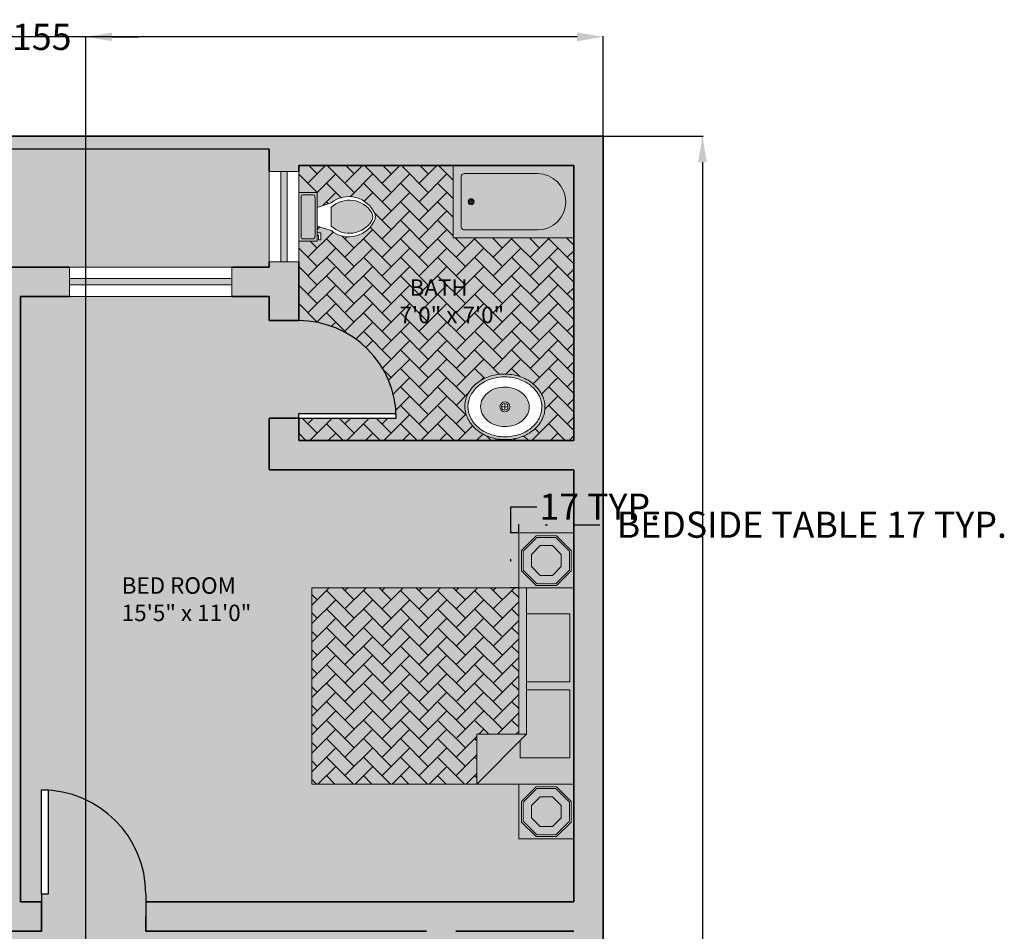
# Model space of a CAD drawing. Units: inches. Extents: x 389 to 971, y 148 to 870.
# Tile 14 of 14: x 670 to 971, y 592 to 870. Entities that reach past the tile are written whole.
import ezdxf

# ---------------------------------------------------------------- set-up
doc = ezdxf.new("R2010")
doc.units = ezdxf.units.IN
doc.header["$MEASUREMENT"] = 0
for name, color, linetype, lineweight in [('A-ANNO-DIMS', 2, 'Continuous', 18), ('A-AREA-IDEN', 7, 'Continuous', 18), ('A-DOOR', 4, 'Continuous', 25), ('A-FLOR-BASE-PATT', 8, 'Continuous', 13), ('A-FLOR-FIXT', 8, 'Continuous', 18), ('A-FLOR-FIXT-PATT', 9, 'Continuous', 13), ('A-FLOR-PATT', 9, 'Continuous', 13), ('A-FURN', 8, 'Continuous', 18), ('A-FURN-PATT', 8, 'Continuous', 13), ('A-GLAZ', 4, 'Continuous', 18), ('A-WALL', 7, 'Continuous', 35), ('C-PROP', 7, 'Continuous', 35), ('L-GRND-BASE-PATT', 8, 'Continuous', 13), ('L-WALL', 7, 'Continuous', 30)]:
    doc.layers.add(name, color=color, linetype=linetype, lineweight=lineweight)
for name, color, linetype, lineweight, true_color in [('A-FURN-SURF-PATT', 9, 'Continuous', 13, 0xd6bdce), ('A-GLAZ-PATT', 251, 'Continuous', 13, 0x6d5f6c), ('A-WALL-PATT', 18, 'Continuous', 13, 0x000000), ('L-GRND-PATT', 39, 'Continuous', 13, 0x603913)]:
    doc.layers.add(name, color=color, linetype=linetype, lineweight=lineweight, true_color=true_color)
doc.styles.get("Standard").update_dxf_attribs({"font": 'arial.ttf'})
doc.dimstyles.get("Standard").update_dxf_attribs({"dimtxt": 8, "dimasz": 8, "dimexe": 0.18, "dimexo": 0.0625, "dimgap": 0.09, "dimtad": 0, "dimtih": 1, "dimtoh": 1, "dimdec": 0, "dimzin": 0, "dimdsep": 46, "dimlunit": 3, "dimtxsty": 'Standard', "dimcen": 0.09, "dimadec": 0, "dimazin": 0, "dimtfac": 1, "dimtdec": 0, "dimtofl": 0, "dimtmove": 0, "dimatfit": 3, "dimfxl": 1, "dimtolj": 1, "dimtzin": 0, "dimarcsym": 0})

# ---------------------------------------------------------------- blocks, each defined once
blk = doc.blocks.new('*U5')
for p, q in [((0, 0), (0, -6)), ((28, 0), (28, -6))]:
    blk.add_line(p, q)
blk.add_lwpolyline([(0, 0), (0, 28), (1.75, 28), (1.75, 0)], close=True)
blk.add_arc((0, 0), 28, 0, 90)
blk = doc.blocks.new('*U3')
for p, q in [((0, 0), (0, -6)), ((-40, 0), (-40, -6))]:
    blk.add_line(p, q)
blk.add_lwpolyline([(0, 0), (0, 40), (-1.75, 40), (-1.75, 0)], close=True)
blk.add_arc((0, 0), 40, 90, 180)
blk = doc.blocks.new('Hot Tub')
for p, q in [((0, 0), (0, 69.12)), ((0, 69.12), (69.12, 69.12)), ((21.601, 65.456), (3.272, 47.128)), ((22.464, 63.396), (5.358, 46.29)), ((47.521, 65.456), (21.601, 65.456)), ((46.656, 63.396), (22.464, 63.396)), ((63.763, 46.29), (46.656, 63.396)), ((65.849, 47.128), (47.521, 65.456)), ((69.12, 69.12), (69.12, 0)), ((26.785, 53.097), (15.788, 42.101)), ((42.337, 53.097), (26.785, 53.097)), ((53.333, 42.101), (42.337, 53.097)), ((3.272, 47.128), (3.272, 21.208)), ((5.358, 46.29), (5.358, 22.098)), ((15.788, 42.101), (15.788, 26.549)), ((53.333, 26.549), (53.333, 42.101)), ((63.763, 22.098), (63.763, 46.29)), ((65.849, 21.208), (65.849, 47.128)), ((15.788, 26.549), (26.785, 15.552)), ((42.337, 15.552), (53.333, 26.549)), ((3.272, 21.208), (21.601, 2.88)), ((5.358, 22.098), (22.464, 4.992)), ((26.785, 15.552), (42.337, 15.552)), ((46.656, 4.992), (63.763, 22.098)), ((47.521, 2.88), (65.849, 21.208)), ((69.12, 0), (0, 0)), ((21.601, 2.88), (47.521, 2.88)), ((22.464, 4.992), (46.656, 4.992))]:
    blk.add_line(p, q)
blk = doc.blocks.new('Toilet - top')
for p, q in [((9.5, -6), (9.5, -2)), ((-8, -8.5), (-8, -8)), ((-7, -8), (-7, -9.5)), ((-4, -8), (-6, -14)), ((4, -8), (6, -14)), ((-10, -8.5), (-8, -8.5)), ((-10, -9.5), (-10, -8.5)), ((-7, -9.5), (-10, -9.5)), ((4, -14), (-4, -14))]:
    blk.add_line(p, q)
blk.add_lwpolyline([(10.5, -8), (10.5, 0), (-10.5, 0), (-10.5, -8)], close=True)
for points in [[(-9.5, -2), (-9.5, -6)], [(8.5, -1), (-8.5, -1)], [(-8.5, -7), (8.5, -7)]]:
    blk.add_lwpolyline(points)
for centre, radius, start, end in [((-8.62, -1.88), 0.884, 81.8699, 188.1301), ((8.62, -1.88), 0.884, 351.8699, 98.1301), ((-8.62, -6.12), 0.884, 171.8699, 278.1301), ((8.62, -6.12), 0.884, 261.8699, 8.1301), ((3.52, -21.58), 12.17, 141.4691, 247.9714), ((4.2, -21.82), 11.33, 136.3677, 238.9468), ((-3.52, -21.58), 12.17, 292.0284, 38.5307), ((-4.2, -21.82), 11.33, 301.053, 43.6321), ((0, -27.88), 4, 245.7318, 294.2682), ((0, -29), 4, 254.8605, 285.1395)]:
    blk.add_arc(centre, radius, start, end)
blk = doc.blocks.new('Bed - Queen')
for p, q in [((0, -80.00003), (0, 0)), ((0, 0), (59.99999, 0)), ((59.99999, 0), (59.99999, -80.00003)), ((7.99999, -1.2), (28.79998, -1.2)), ((7.99999, -14.4), (7.99999, -1.2)), ((28.79998, -1.2), (28.79998, -14.4)), ((31.19999, -1.2), (51.99999, -1.2)), ((31.19999, -14.4), (31.19999, -1.2)), ((51.99999, -1.2), (51.99999, -16.4)), ((0, -14.4), (44.8, -14.4)), ((59.99999, -29.6), (44.8, -14.4)), ((44.8, -14.4), (44.8, -29.6)), ((44.8, -16.8), (0, -16.8)), ((51.99999, -16.4), (46.79936, -16.4)), ((44.8, -29.6), (59.99999, -29.6)), ((59.99999, -80.00003), (0, -80.00003))]:
    blk.add_line(p, q)
blk = doc.blocks.new('Sink - Oval top')
for p, q in [((-1, 0), (1, 0)), ((0, 1), (0, -1))]:
    blk.add_line(p, q)
for points in [[(-12.23, 0.39, 0.117634), (-11.46, -3.36, 0.104469), (-8.88, -6.8, 0.090016), (-5.08, -9.07, 0.08192), (-0.32, -10.02, 0.08192), (4.49, -9.38, 0.090016), (8.42, -7.36, 0.104469), (11.22, -4.09, 0.117634), (12.23, -0.39, 0.117634), (11.46, 3.36, 0.104469), (8.88, 6.8, 0.090016), (5.08, 9.07, 0.08192), (0.32, 10.02, 0.08192), (-4.49, 9.38, 0.090016), (-8.42, 7.36, 0.104469), (-11.22, 4.09, 0.117634)], [(-11.29, 0.16, 0.118622), (-10.52, -3.25, 0.104678), (-8.07, -6.36, 0.089562), (-4.54, -8.37, 0.081185), (-0.13, -9.15, 0.081185), (4.3, -8.49, 0.089562), (7.89, -6.58, 0.104678), (10.42, -3.55, 0.118622), (11.29, -0.16, 0.118622), (10.52, 3.25, 0.104678), (8.07, 6.36, 0.089562), (4.54, 8.37, 0.081185), (0.13, 9.15, 0.081185), (-4.3, 8.49, 0.089562), (-7.89, 6.58, 0.104678), (-10.42, 3.55, 0.118622)], [(-7.42, 0.08, 0.118283), (-6.91, -2.17, 0.104607), (-5.29, -4.21, 0.089718), (-2.97, -5.53, 0.081436), (-0.07, -6.04, 0.081436), (2.84, -5.59, 0.089718), (5.2, -4.33, 0.104607), (6.86, -2.32, 0.118283), (7.42, -0.08, 0.118283), (6.91, 2.17, 0.104607), (5.29, 4.21, 0.089718), (2.97, 5.53, 0.081436), (0.07, 6.04, 0.081436), (-2.84, 5.59, 0.089718), (-5.2, 4.33, 0.104607), (-6.86, 2.32, 0.118283)]]:
    blk.add_lwpolyline(points, format="xyb", close=True)
for radius in [1.5, 1]:
    blk.add_circle((0, 0), radius)
blk = doc.blocks.new('Bath Tub - 26 x 60 in.')
for p, q in [((8, -18), (10, -18)), ((9, -17), (9, -19))]:
    blk.add_line(p, q)
blk.add_lwpolyline([(0, -36), (0, 0), (60, 0), (60, -36)], close=True)
for points in [[(6, -4), (42, -4)], [(4, -30), (4, -6)], [(42, -32), (6, -32)]]:
    blk.add_lwpolyline(points)
for radius in [1.5, 1]:
    blk.add_circle((9, -18), radius)
for centre, radius, start, end in [((5.75, -5.75), 1.77, 81.8699, 188.1301), ((42, -18), 14, 270, 90), ((5.75, -30.25), 1.77, 171.8699, 278.1301)]:
    blk.add_arc(centre, radius, start, end)
blk = doc.blocks.new('*D22')
at = {"layer": 'A-ANNO-DIMS', "color": 0, "lineweight": -2, "transparency": 16777216}
for p, q in [((822.48, 713.45), (822.48, 716.08)), ((830.48, 715.9), (831.22, 715.9)), ((839.22, 713.45), (839.22, 716.08)), ((839.22, 715.9), (847.22, 715.9))]:
    blk.add_line(p, q, dxfattribs=at)
at = {"layer": 'A-ANNO-DIMS', "color": 0, "transparency": 16777216}
for points in [[(830.48, 717.23), (830.48, 714.56), (822.48, 715.9)], [(831.22, 717.23), (831.22, 714.56), (839.22, 715.9)]]:
    blk.add_solid(points, dxfattribs=at)
at = {"layer": 'Defpoints', "color": 0, "transparency": 16777216}
for p in [(839.22, 715.9), (822.48, 713.39), (839.22, 713.39)]:
    blk.add_point(p, dxfattribs=at)
at = {"layer": 'A-ANNO-DIMS', "color": 0, "transparency": 16777216, "insert": (911.94, 715.9), "char_height": 8, "attachment_point": 5}
blk.add_mtext('\\A1;BEDSIDE TABLE 17 TYP.', dxfattribs=at)
blk = doc.blocks.new('*D23')
at = {"layer": 'A-ANNO-DIMS', "color": 0, "lineweight": -2, "transparency": 16777216}
for p, q in [((819.96, 713.39), (819.96, 721.39)), ((819.96, 721.39), (827.96, 721.39)), ((822.41, 713.39), (819.78, 713.39)), ((819.96, 704.64), (819.96, 705.39)), ((822.41, 696.64), (819.78, 696.64))]:
    blk.add_line(p, q, dxfattribs=at)
at = {"layer": 'A-ANNO-DIMS', "color": 0, "transparency": 16777216}
for points in [[(818.63, 705.39), (821.3, 705.39), (819.96, 713.39)], [(818.63, 704.64), (821.3, 704.64), (819.96, 696.64)]]:
    blk.add_solid(points, dxfattribs=at)
at = {"layer": 'Defpoints', "color": 0, "transparency": 16777216}
for p in [(819.96, 713.39), (822.48, 713.39), (822.48, 696.64)]:
    blk.add_point(p, dxfattribs=at)
at = {"layer": 'A-ANNO-DIMS', "color": 0, "transparency": 16777216, "insert": (847.15, 721.39), "char_height": 8, "attachment_point": 5}
blk.add_mtext('\\A1;17 TYP.', dxfattribs=at)
blk = doc.blocks.new('*D46')
at = {"layer": 'A-ANNO-DIMS', "color": 0, "lineweight": -2, "transparency": 16777216}
for p, q in [((468.22, 794.71), (468.22, 865.15)), ((476.22, 864.97), (649.3, 864.97)), ((840.22, 864.97), (667.13, 864.97)), ((848.22, 834.71), (848.22, 865.15))]:
    blk.add_line(p, q, dxfattribs=at)
at = {"layer": 'A-ANNO-DIMS', "color": 0, "transparency": 16777216}
for points in [[(476.22, 866.3), (476.22, 863.64), (468.22, 864.97)], [(840.22, 866.3), (840.22, 863.64), (848.22, 864.97)]]:
    blk.add_solid(points, dxfattribs=at)
at = {"layer": 'Defpoints', "color": 0, "transparency": 16777216}
for p in [(848.22, 864.97), (848.22, 834.64), (468.22, 794.64)]:
    blk.add_point(p, dxfattribs=at)
at = {"layer": 'A-ANNO-DIMS', "color": 0, "transparency": 16777216, "insert": (658.22, 864.97), "char_height": 8, "attachment_point": 5}
blk.add_mtext('\\A1;380', dxfattribs=at)
blk = doc.blocks.new('*D47')
at = {"layer": 'A-ANNO-DIMS', "color": 0, "lineweight": -2, "transparency": 16777216}
for p, q in [((848.28, 834.64), (878.72, 834.64)), ((878.54, 826.64), (878.54, 564.32)), ((878.54, 293.64), (878.54, 555.97)), ((839.28, 285.64), (878.72, 285.64))]:
    blk.add_line(p, q, dxfattribs=at)
at = {"layer": 'A-ANNO-DIMS', "color": 0, "transparency": 16777216}
for points in [[(877.21, 826.64), (879.87, 826.64), (878.54, 834.64)], [(877.21, 293.64), (879.87, 293.64), (878.54, 285.64)]]:
    blk.add_solid(points, dxfattribs=at)
at = {"layer": 'Defpoints', "color": 0, "transparency": 16777216}
for p in [(848.22, 834.64), (878.54, 834.64), (839.22, 285.64)]:
    blk.add_point(p, dxfattribs=at)
at = {"layer": 'A-ANNO-DIMS', "color": 0, "transparency": 16777216, "insert": (878.54, 560.14), "char_height": 8, "attachment_point": 5}
blk.add_mtext('\\A1;549', dxfattribs=at)
blk = doc.blocks.new('*D52')
at = {"layer": 'A-ANNO-DIMS', "color": 0, "lineweight": -2, "transparency": 16777216}
for p, q in [((640.06, 864.97), (632.06, 864.97)), ((648.06, 388.98), (648.06, 865.15)), ((690.22, 388.98), (690.22, 865.15)), ((698.22, 864.97), (706.22, 864.97))]:
    blk.add_line(p, q, dxfattribs=at)
at = {"layer": 'A-ANNO-DIMS', "color": 0, "transparency": 16777216}
for points in [[(640.06, 866.3), (640.06, 863.64), (648.06, 864.97)], [(698.22, 866.3), (698.22, 863.64), (690.22, 864.97)]]:
    blk.add_solid(points, dxfattribs=at)
at = {"layer": 'Defpoints', "color": 0, "transparency": 16777216}
for p in [(690.22, 864.97), (648.06, 388.92), (690.22, 388.92)]:
    blk.add_point(p, dxfattribs=at)
at = {"layer": 'A-ANNO-DIMS', "color": 0, "transparency": 16777216, "insert": (669.14, 864.97), "char_height": 8, "attachment_point": 5}
blk.add_mtext('\\A1;42.155', dxfattribs=at)

msp = doc.modelspace()

# ---------------------------------------------------------------- hatches: boundary and pattern name
at = {"layer": 'A-FLOR-BASE-PATT'}
h = msp.add_hatch(color=256, dxfattribs=at)
h.dxf.hatch_style = 1
h.paths.add_polyline_path([(823.2691, 760.9857, -0.09001579), (827.065, 758.7169, -0.10446928), (829.6509, 755.2753, -0.11763426), (830.42, 751.5192, -0.11763426), (829.4106, 747.8203, -0.10446928), (826.6086, 744.5523, -0.09001579), (822.6745, 742.5326, -0.07381843), (818.3437, 741.8898), (839.216, 741.6445), (839.216, 803.5176), (802.3378, 803.5176), (802.3378, 825.6445), (755.216, 825.6445), (755.216, 823.8175), (755.216, 817.4527), (760.891, 817.4527), (760.891, 812.8418), (765.1472, 814.2605, -0.50132349), (778.5269, 810.7453, -0.13289091), (778.5269, 809.2632, -0.50131678), (765.1474, 805.748), (760.891, 807.1668), (760.891, 805.0386), (761.9551, 805.0386), (761.9551, 802.9105), (760.891, 802.9105), (760.891, 802.5558), (755.216, 802.5558), (755.216, 796.191), (755.216, 778.2586, -0.40115902), (784.9563, 749.7633), (784.9849, 749.7633), (784.9849, 748.4596), (755.216, 748.4596), (755.216, 741.6445), (818.3437, 741.8898, -0.09003216), (813.1035, 742.841, -0.09001579), (809.3075, 745.1098, -0.10446928), (806.7217, 748.5514, -0.11763426), (805.9526, 752.3075, -0.11763426), (806.9619, 756.0064, -0.10446928), (809.764, 759.2744, -0.09001579), (813.6981, 761.2941, -0.08191995), (818.509, 761.9292, -0.08191995)])
h.paths.add_polyline_path([(784.4177, 774.7212), (817.5794, 774.7212), (817.5794, 793.4478), (784.4177, 793.4478)], flags=24)
h = msp.add_hatch(color=256, dxfattribs=at)
h.dxf.hatch_style = 1
h.paths.add_polyline_path([(670.216, 600.6445), (676.6391, 600.6445), (676.6391, 602.9755), (676.6391, 634.8535), (678.6314, 634.8535), (678.6314, 634.7912, -0.39601219), (708.5171, 602.9755), (708.5171, 600.6445), (839.216, 600.6445), (839.216, 619.9039), (822.4754, 619.9039), (822.4754, 636.6445), (759.216, 636.6445), (759.216, 696.6445), (822.4754, 696.6445), (822.4754, 713.3852), (839.216, 713.3852), (839.216, 732.6445), (746.216, 732.6445), (746.216, 748.4596), (755.1859, 748.4596), (755.1859, 749.7633), (784.9563, 749.7633, 0.40145271), (755.1859, 778.2586), (750.716, 778.2586), (746.216, 778.2905), (746.216, 785.6445), (734.7772, 785.6445), (670.216, 785.6445)])
h.paths.add_polyline_path([(699.1372, 683.5869), (740.0971, 683.5869), (740.0971, 702.3135), (699.1372, 702.3135)], flags=24)
h = msp.add_hatch(color=256, dxfattribs=at)
h.dxf.hatch_style = 1
h.paths.add_polyline_path([(634.6594, 428.4021), (634.6594, 427.0792), (634.6305, 427.0792, -0.40145271), (604.4225, 398.1652), (604.0817, 398.1199, -0.40145271), (632.0195, 371.3788), (632.0462, 371.3788), (632.0462, 370.1554), (604.387, 370.1554), (604.387, 366.7191), (640.0296, 366.7191), (640.0296, 321.4969, 1), (647.061, 321.4969), (647.061, 412.9189), (690.216, 412.9189), (690.216, 416.0006), (694.716, 416.0006), (702.2145, 416.0006, 0.39601219), (737.1392, 448.8066), (702.2145, 448.8066), (702.2145, 450.9936), (694.716, 450.9936), (690.216, 450.9936), (690.216, 466.6012), (708.7881, 466.6012), (708.7881, 462.1012), (784.6145, 462.1012), (784.6145, 466.6012), (794.216, 466.6012), (794.216, 591.6445), (708.5171, 591.6445), (708.5171, 596.1445), (708.5171, 602.9755, 0.39601219), (678.6314, 634.7912), (678.6314, 602.9755), (676.6391, 602.9755), (676.6391, 596.1445), (676.6391, 591.6445), (661.216, 591.6445), (661.216, 632.6445), (653.109, 632.6445), (653.109, 641.6445), (653.109, 642.1751), (651.6417, 642.1751), (651.6417, 675.6801, 0.40145271), (619.5719, 642.1751), (619.5719, 637.1445), (619.5147, 632.6445), (604.387, 632.6445), (604.387, 545.7317), (595.3894, 545.7317), (595.3894, 544.4199), (565.4338, 544.4199, 0.40145271), (595.3894, 515.7475), (599.887, 515.7475), (604.387, 515.7271), (604.387, 428.4021)])
h.paths.add_polyline_path([(721.8003, 493.9292), (725.0899, 493.9292), (725.0899, 493.075), (751.4065, 493.075), (751.4065, 493.9292), (754.6961, 493.9292), (754.6961, 479.6744, -0.26666697), (721.8003, 479.6744)], flags=16)
h.paths.add_polyline_path([(720.6421, 516.0583), (720.6421, 545.0393), (753.5806, 545.0393), (753.5806, 516.0583)], flags=16)
h.paths.add_polyline_path([(722.6421, 518.0583), (722.6421, 543.0393), (751.5806, 543.0393), (751.5806, 518.0583)], flags=0)
h.paths.add_polyline_path([(763.7396, 488.5801), (763.7822, 488.1156), (764.1436, 488.1761)], flags=16)
h.paths.add_polyline_path([(777.9011, 479.7417), (778.0475, 480.1886), (777.4745, 480.275)], flags=16)
h.paths.add_polyline_path([(762.3329, 503.5919), (762.3329, 507.1718), (763.2624, 507.1718), (763.2624, 550.1306), (762.3329, 550.1306), (762.3329, 553.7105), (777.8458, 553.7105, -0.19047621), (777.8458, 503.5919)], flags=16)
h.paths.add_polyline_path([(721.6097, 567.2898), (721.6097, 581.7362, -0.26666697), (754.9475, 581.7362), (754.9475, 567.2898), (751.6137, 567.2898), (751.6137, 568.1555), (724.9435, 568.1555), (724.9435, 567.2898)], flags=16)
h.paths.add_polyline_path([(774.6347, 521.4914), (774.6347, 535.811), (778.6837, 535.811, -0.04962821), (778.6837, 521.4914)], flags=0)
h.paths.add_polyline_path([(764.6624, 576.8996), (764.7454, 576.4742), (765.0717, 576.4903)], flags=16)
h.paths.add_polyline_path([(777.2772, 570.3652), (777.4444, 570.8756), (776.7899, 570.9743)], flags=16)
h.paths.add_polyline_path([(644.2892, 516.9956), (685.2491, 516.9956), (685.2491, 535.7223), (644.2892, 535.7223)], flags=24)
h = msp.add_hatch(color=256, dxfattribs=at)
h.dxf.hatch_style = 1
h.paths.add_polyline_path([(839.216, 591.6445), (803.216, 591.6445), (803.216, 466.6012), (839.216, 466.6012)])
at = {"layer": 'A-FLOR-FIXT-PATT'}
h = msp.add_hatch(color=256, dxfattribs=at)
h.dxf.hatch_style = 1
h.paths.add_polyline_path([(804.7964, 807.2054, 0.50000012), (806.0257, 805.9762), (828.1526, 805.9762, 1), (828.1526, 823.186), (806.0257, 823.186, 0.50000012), (804.7964, 821.9567)], flags=16)
h.paths.add_polyline_path([(839.216, 803.5176), (839.216, 825.6445), (802.3378, 825.6445), (802.3378, 803.5176)])
h.paths.add_polyline_path([(806.9476, 814.5811, -1), (808.7915, 814.5811, -1)], flags=0)
h.paths.add_polyline_path([(807.2549, 814.5811, -1), (808.4842, 814.5811, -1)], flags=0)
h = msp.add_hatch(color=256, dxfattribs=at)
h.dxf.hatch_style = 1
h.paths.add_polyline_path([(806.0257, 823.186, 0.50000012), (804.7964, 821.9567), (804.7964, 807.2054, 0.50000012), (806.0257, 805.9762), (828.1526, 805.9762, 1), (828.1526, 823.186)])
h.paths.add_polyline_path([(806.9476, 814.5811, -1), (808.7915, 814.5811, -1)], flags=16)
h.paths.add_polyline_path([(807.2549, 814.5811, -1), (808.4842, 814.5811, -1)], flags=0)
h = msp.add_hatch(color=256, dxfattribs=at)
h.dxf.hatch_style = 1
h.paths.add_polyline_path([(760.891, 817.4527), (755.216, 817.4527), (755.216, 802.5558), (760.891, 802.5558)])
h.paths.add_polyline_path([(765.1473, 812.8418, -0.4800795), (777.5777, 811.1705, -0.21500378), (777.5777, 808.838, -0.48007965), (765.1473, 807.1668)], flags=17)
h = msp.add_hatch(color=256, dxfattribs=at)
h.dxf.hatch_style = 1
h.paths.add_polyline_path([(829.6509, 755.2753, 0.10446928), (827.065, 758.7169, 0.09001579), (823.2691, 760.9857, 0.08191995), (818.509, 761.9292, 0.08191995), (813.6981, 761.2941, 0.09001579), (809.764, 759.2744, 0.10446928), (806.9619, 756.0064, 0.11763426), (805.9526, 752.3075, 0.11763426), (806.7217, 748.5514, 0.10446928), (809.3075, 745.1098, 0.09001579), (813.1035, 742.841, 0.08191995), (817.8636, 741.8975, 0.08191995), (822.6745, 742.5326, 0.09001579), (826.6086, 744.5523, 0.10446928), (829.4106, 747.8203, 0.11763426), (830.42, 751.5192, 0.11763426)])
h.paths.add_polyline_path([(829.4726, 751.7543, -0.1186217), (828.6063, 748.3651, -0.10467817), (826.0757, 745.3298, -0.08956207), (822.4864, 743.4218, -0.0811847), (818.0573, 742.7618, -0.0811847), (813.6486, 743.5464, -0.08956207), (810.1145, 745.5547, -0.10467817), (807.6704, 748.6602, -0.1186217), (806.9, 752.0724, -0.1186217), (807.7662, 755.4616, -0.10467817), (810.2969, 758.4969, -0.08956207), (813.8862, 760.4049, -0.0811847), (818.3153, 761.0649, -0.0811847), (822.724, 760.2803, -0.08956207), (826.2581, 758.272, -0.10467817), (828.7022, 755.1665, -0.1186217)], flags=16)
h.paths.add_polyline_path([(825.6067, 751.8304, -0.11828257), (825.0432, 749.592, -0.10460746), (823.3856, 747.586, -0.08971796), (821.0285, 746.3203, -0.08143608), (818.1188, 745.8765, -0.08143608), (815.2197, 746.3852, -0.08971796), (812.8915, 747.7034, -0.10460746), (811.2792, 749.7459, -0.11828257), (810.7658, 751.9963, -0.11828257), (811.3294, 754.2347, -0.10460746), (812.987, 756.2407, -0.08971796), (815.3441, 757.5064, -0.08143608), (818.2538, 757.9502, -0.08143608), (821.1529, 757.4415, -0.08971796), (823.4811, 756.1233, -0.10460746), (825.0934, 754.0808, -0.11828257)], flags=0)
h.paths.add_polyline_path([(819.6863, 751.9133, -1), (816.6863, 751.9133, -1)], flags=0)
h.paths.add_polyline_path([(819.1863, 751.9133, -1), (817.1863, 751.9133, -1)], flags=0)
h = msp.add_hatch(color=256, dxfattribs=at)
h.dxf.hatch_style = 1
h.paths.add_polyline_path([(825.0934, 754.0808, 0.10460746), (823.4811, 756.1233, 0.08971796), (821.1529, 757.4415, 0.08143608), (818.2538, 757.9502, 0.08143608), (815.3441, 757.5064, 0.08971796), (812.987, 756.2407, 0.10460746), (811.3294, 754.2347, 0.11828257), (810.7658, 751.9963, 0.11828257), (811.2792, 749.7459, 0.10460746), (812.8915, 747.7034, 0.08971796), (815.2197, 746.3852, 0.08143608), (818.1188, 745.8765, 0.08143608), (821.0285, 746.3203, 0.08971796), (823.3856, 747.586, 0.10460746), (825.0432, 749.592, 0.11828257), (825.6067, 751.8304, 0.11828257)])
h.paths.add_polyline_path([(819.6863, 751.9133, -1), (816.6863, 751.9133, -1)], flags=16)
h.paths.add_polyline_path([(819.1863, 751.9133, -1), (817.1863, 751.9133, -1)], flags=0)
at = {"layer": 'A-FLOR-PATT'}
h = msp.add_hatch(dxfattribs=at)
h.set_pattern_fill('AR-HBONE', color=256)
h.paths.add_polyline_path([(809.764, 759.2744, -0.09001579), (813.6981, 761.2941, -0.08191995), (818.509, 761.9292, -0.08191995), (823.2691, 760.9857, -0.09001579), (827.065, 758.7169, -0.10446928), (829.6509, 755.2753, -0.11763426), (830.42, 751.5192, -0.11763426), (829.4106, 747.8203, -0.10446928), (826.6086, 744.5523, -0.09001579), (822.6745, 742.5326, -0.07381843), (818.3437, 741.8898), (839.216, 741.6445), (839.216, 803.5176), (802.3378, 803.5176), (802.3378, 825.6445), (755.216, 825.6445), (755.216, 823.8175), (755.216, 817.4527), (760.891, 817.4527), (760.891, 812.8418), (765.1472, 814.2605, -0.50132349), (778.5269, 810.7453, -0.13289091), (778.5269, 809.2632, -0.50131678), (765.1474, 805.748), (760.891, 807.1668), (760.891, 805.0386), (761.9551, 805.0386), (761.9551, 802.9105), (760.891, 802.9105), (760.891, 802.5558), (755.216, 802.5558), (755.216, 796.191), (755.216, 778.2586, -0.40115902), (784.9563, 749.7633), (784.9849, 749.7633), (784.9849, 748.4596), (755.216, 748.4596), (755.216, 741.6445), (818.3437, 741.8898, -0.09003216), (813.1035, 742.841, -0.09001579), (809.3075, 745.1098, -0.10446928), (806.7217, 748.5514, -0.11763426), (805.9526, 752.3075, -0.11763426), (806.9619, 756.0064, -0.10446928)])
h.paths.add_polyline_path([(784.4177, 774.7212), (817.5794, 774.7212), (817.5794, 793.4478), (784.4177, 793.4478)], flags=24)
at = {"layer": 'A-FURN-PATT'}
h = msp.add_hatch(dxfattribs=at)
h.set_pattern_fill('AR-HBONE', color=256)
h.paths.add_polyline_path([(759.216, 636.6445), (809.616, 636.6445), (809.616, 651.8445), (822.416, 651.8445), (822.416, 696.6445), (759.216, 696.6445)])
at = {"layer": 'A-FURN-SURF-PATT'}
h = msp.add_hatch(color=256, dxfattribs=at)
h.dxf.hatch_style = 1
h.paths.add_polyline_path([(839.216, 713.3852), (822.4754, 713.3852), (822.4754, 696.6445), (839.216, 696.6445)])
h.paths.add_polyline_path([(823.2678, 701.781), (823.2678, 708.0588), (827.7071, 712.4978), (833.9848, 712.4978), (838.4238, 708.0588), (838.4238, 701.781), (833.9848, 697.342), (827.7071, 697.342)], flags=16)
h.paths.add_polyline_path([(823.7731, 701.9966), (823.7731, 707.8558), (827.9161, 711.9988), (833.7753, 711.9988), (837.9186, 707.8558), (837.9186, 701.9966), (833.7753, 697.8536), (827.9161, 697.8536)], flags=0)
h.paths.add_polyline_path([(826.2992, 703.0746), (826.2992, 706.8412), (828.9626, 709.5044), (832.7293, 709.5044), (835.3925, 706.8412), (835.3925, 703.0746), (832.7293, 700.4112), (828.9626, 700.4112)], flags=0)
h = msp.add_hatch(color=256, dxfattribs=at)
h.dxf.hatch_style = 1
h.paths.add_polyline_path([(826.2992, 703.0746), (828.9626, 700.4112), (832.7293, 700.4112), (835.3925, 703.0746), (835.3925, 706.8412), (832.7293, 709.5044), (828.9626, 709.5044), (826.2992, 706.8412)], flags=16)
h.paths.add_polyline_path([(827.9161, 697.8536), (833.7753, 697.8536), (837.9186, 701.9966), (837.9186, 707.8558), (833.7753, 711.9988), (827.9161, 711.9988), (823.7731, 707.8558), (823.7731, 701.9966)])
h = msp.add_hatch(color=256, dxfattribs=at)
h.dxf.hatch_style = 1
h.paths.add_polyline_path([(826.2992, 706.8412), (826.2992, 703.0746), (828.9626, 700.4112), (832.7293, 700.4112), (835.3925, 703.0746), (835.3925, 706.8412), (832.7293, 709.5044), (828.9626, 709.5044)])
h = msp.add_hatch(color=256, dxfattribs=at)
h.dxf.hatch_style = 1
h.paths.add_polyline_path([(759.216, 696.6445), (759.216, 636.6445), (809.616, 636.6445), (809.616, 651.8445), (822.416, 651.8445), (822.416, 696.6445)])
h = msp.add_hatch(color=256, dxfattribs=at)
h.dxf.hatch_style = 1
h.paths.add_polyline_path([(838.016, 688.6445), (838.016, 667.8445), (824.816, 667.8445), (824.816, 665.4445), (838.016, 665.4445), (838.016, 644.6445), (822.816, 644.6445), (822.816, 649.8445), (809.616, 636.6445), (839.216, 636.6445), (839.216, 696.6445), (824.816, 696.6445), (824.816, 688.6445)])
h = msp.add_hatch(color=256, dxfattribs=at)
h.dxf.hatch_style = 1
h.paths.add_polyline_path([(822.416, 651.8445), (824.816, 651.8445), (824.816, 696.6445), (822.416, 696.6445)])
h = msp.add_hatch(color=256, dxfattribs=at)
h.dxf.hatch_style = 1
h.paths.add_polyline_path([(838.016, 688.6445), (824.816, 688.6445), (824.816, 667.8445), (838.016, 667.8445)])
h = msp.add_hatch(color=256, dxfattribs=at)
h.dxf.hatch_style = 1
h.paths.add_polyline_path([(824.816, 651.8445), (822.816, 649.8445), (822.816, 644.6445), (838.016, 644.6445), (838.016, 665.4445), (824.816, 665.4445)])
h = msp.add_hatch(color=256, dxfattribs=at)
h.dxf.hatch_style = 1
h.paths.add_polyline_path([(809.616, 636.6445), (824.816, 651.8445), (809.616, 651.8445)])
h = msp.add_hatch(color=256, dxfattribs=at)
h.dxf.hatch_style = 1
h.paths.add_polyline_path([(839.216, 636.6445), (822.4754, 636.6445), (822.4754, 619.9039), (839.216, 619.9039)])
h.paths.add_polyline_path([(823.2678, 625.0404), (823.2678, 631.3181), (827.7071, 635.7571), (833.9848, 635.7571), (838.4238, 631.3181), (838.4238, 625.0404), (833.9848, 620.6014), (827.7071, 620.6014)], flags=16)
h.paths.add_polyline_path([(823.7731, 625.2559), (823.7731, 631.1152), (827.9161, 635.2582), (833.7753, 635.2582), (837.9186, 631.1152), (837.9186, 625.2559), (833.7753, 621.1129), (827.9161, 621.1129)], flags=0)
h.paths.add_polyline_path([(826.2992, 626.3339), (826.2992, 630.1006), (828.9626, 632.7638), (832.7293, 632.7638), (835.3925, 630.1006), (835.3925, 626.3339), (832.7293, 623.6705), (828.9626, 623.6705)], flags=0)
h = msp.add_hatch(color=256, dxfattribs=at)
h.dxf.hatch_style = 1
h.paths.add_polyline_path([(835.3925, 626.3339), (835.3925, 630.1006), (832.7293, 632.7638), (828.9626, 632.7638), (826.2992, 630.1006), (826.2992, 626.3339), (828.9626, 623.6705), (832.7293, 623.6705)], flags=16)
h.paths.add_polyline_path([(837.9186, 631.1152), (833.7753, 635.2582), (827.9161, 635.2582), (823.7731, 631.1152), (823.7731, 625.2559), (827.9161, 621.1129), (833.7753, 621.1129), (837.9186, 625.2559)])
h = msp.add_hatch(color=256, dxfattribs=at)
h.dxf.hatch_style = 1
h.paths.add_polyline_path([(832.7293, 623.6705), (835.3925, 626.3339), (835.3925, 630.1006), (832.7293, 632.7638), (828.9626, 632.7638), (826.2992, 630.1006), (826.2992, 626.3339), (828.9626, 623.6705)])
at = {"layer": 'A-GLAZ-PATT'}
h = msp.add_hatch(color=256, dxfattribs=at)
h.dxf.hatch_style = 1
h.paths.add_polyline_path([(751.716, 823.8175), (749.716, 823.8175), (749.716, 796.191), (751.716, 796.191)])
h = msp.add_hatch(color=256, dxfattribs=at)
h.dxf.hatch_style = 1
h.paths.add_polyline_path([(734.7772, 789.1445), (734.7772, 791.1445), (685.2392, 791.1445), (685.2392, 789.1445)])
at = {"layer": 'A-WALL-PATT'}
h = msp.add_hatch(color=256, dxfattribs=at)
h.dxf.hatch_style = 1
h.paths.add_polyline_path([(432.216, 434.6445), (436.3673, 434.6445), (436.3673, 443.6445), (432.216, 443.6445), (432.216, 830.6445), (746.216, 830.6445), (746.216, 823.8175), (755.216, 823.8175), (755.216, 825.6445), (839.216, 825.6445), (839.216, 803.5176), (839.216, 741.6445), (755.216, 741.6445), (755.216, 748.4596), (755.1859, 748.4596), (750.716, 748.4596), (746.216, 748.4596), (746.216, 732.6445), (839.216, 732.6445), (839.216, 600.6445), (708.5171, 600.6445), (708.5171, 596.1445), (708.5171, 591.6445), (794.216, 591.6445), (794.216, 587.4291), (803.216, 587.4291), (803.216, 591.6445), (839.216, 591.6445), (839.216, 466.6012), (803.216, 466.6012), (803.216, 471.0309), (794.216, 471.0309), (794.216, 466.6012), (784.6145, 466.6012), (784.6145, 457.6012), (839.216, 457.6012), (839.216, 447.6445), (839.216, 294.6445), (810.0514, 294.6445), (810.0514, 285.6445), (839.216, 285.6445), (839.216, 238.6445), (590.216, 238.6445), (590.216, 234.6445), (848.216, 234.6445), (848.216, 834.6445), (428.216, 834.6445), (428.216, 234.6445), (437.216, 234.6445), (437.216, 243.6445), (432.216, 243.6445)])
h = msp.add_hatch(color=256, dxfattribs=at)
h.dxf.hatch_style = 1
h.paths.add_polyline_path([(661.216, 785.6445), (661.216, 641.6445), (653.109, 641.6445), (653.109, 637.1445), (653.109, 632.6445), (661.216, 632.6445), (661.216, 591.6445), (676.6391, 591.6445), (676.6391, 600.6445), (670.216, 600.6445), (670.216, 785.6445), (685.2392, 785.6445), (685.2392, 794.6445), (662.4125, 794.6445), (606.2724, 794.6445), (606.2724, 785.6445), (616.7487, 785.6445)])
h = msp.add_hatch(color=256, dxfattribs=at)
h.dxf.hatch_style = 1
h.paths.add_polyline_path([(755.216, 796.191), (746.216, 796.191), (746.216, 794.6445), (734.7772, 794.6445), (734.7772, 785.6445), (746.216, 785.6445), (746.216, 778.2905), (755.216, 778.2905)])
at = {"layer": 'L-GRND-BASE-PATT'}
h = msp.add_hatch(color=256, dxfattribs=at)
h.dxf.hatch_style = 1
h.paths.add_polyline_path([(468.216, 560.6445), (502.387, 560.6445), (502.387, 585.4344), (502.387, 613.354), (502.387, 632.6445), (468.216, 632.6445), (468.216, 651.2738), (468.216, 699.1491), (468.216, 728.9805), (468.216, 777.4428), (468.216, 794.6445), (534.7176, 794.6445), (606.2724, 794.6445), (685.2392, 794.6445), (734.7772, 794.6445), (746.216, 794.6445), (746.216, 796.191), (746.216, 823.8175), (746.216, 830.6445), (432.216, 830.6445), (432.216, 443.6445), (468.216, 443.6445), (468.216, 452.1978), (468.216, 490.1255), (468.216, 508.3496), (468.216, 543.0462)])
h.paths.add_polyline_path([(456.8918, 600.1849), (456.8918, 677.4216), (446.55, 677.4216), (446.55, 600.1849)], flags=24)
h.paths.add_polyline_path([(573.4326, 807.2886), (651.063, 807.2886), (651.063, 817.6304), (573.4326, 817.6304)], flags=24)
at = {"layer": 'L-GRND-PATT'}
h = msp.add_hatch(dxfattribs=at)
h.set_pattern_fill('EARTH', color=256, angle=45)
h.set_pattern_definition([(45, (0, 0), (0, 8.980256), [6.35, -6.35]), (45, (-1.684, 1.684), (0, 8.980256), [6.35, -6.35]), (45, (-3.3676, 3.3676), (0, 8.980256), [6.35, -6.35]), (135, (-3.3676, 4.49), (-8.980256, 0), [6.35, -6.35]), (135, (-1.684, 6.174), (-8.980256, 0), [6.35, -6.35]), (135, (0, 7.858), (-8.980256, 0), [6.35, -6.35])])
h.paths.add_polyline_path([(468.216, 560.6445), (502.387, 560.6445), (502.387, 585.4344), (502.387, 613.354), (502.387, 632.6445), (468.216, 632.6445), (468.216, 651.2738), (468.216, 699.1491), (468.216, 728.9805), (468.216, 777.4428), (468.216, 794.6445), (534.7176, 794.6445), (606.2724, 794.6445), (685.2392, 794.6445), (734.7772, 794.6445), (746.216, 794.6445), (746.216, 796.191), (746.216, 823.8175), (746.216, 830.6445), (432.216, 830.6445), (432.216, 443.6445), (468.216, 443.6445), (468.216, 452.1978), (468.216, 490.1255), (468.216, 508.3496), (468.216, 543.0462)])
h.paths.add_polyline_path([(456.8918, 600.1849), (456.8918, 677.4216), (446.55, 677.4216), (446.55, 600.1849)], flags=24)
h.paths.add_polyline_path([(573.4326, 807.2886), (651.063, 807.2886), (651.063, 817.6304), (573.4326, 817.6304)], flags=24)

# ---------------------------------------------------------------- linework, layer by layer
at = {"layer": 'A-GLAZ'}
for p, q in [((755.216, 823.8175), (746.216, 823.8175)), ((746.216, 823.8175), (746.216, 796.191)), ((749.716, 823.8175), (749.716, 796.191)), ((751.716, 823.8175), (751.716, 796.191)), ((755.216, 823.8175), (755.216, 796.191)), ((662.4125, 794.6445), (734.7772, 794.6445)), ((685.2392, 785.6445), (685.2392, 794.6445)), ((734.7772, 785.6445), (734.7772, 794.6445)), ((734.7772, 794.6445), (734.7772, 785.6445)), ((746.216, 796.191), (755.216, 796.191)), ((685.2392, 791.1445), (734.7772, 791.1445)), ((685.2392, 789.1445), (734.7772, 789.1445)), ((670.216, 785.6445), (734.7772, 785.6445))]:
    msp.add_line(p, q, dxfattribs=at)
at = {"layer": 'A-WALL'}
for p, q in [((746.216, 823.8175), (746.216, 830.6445)), ((839.216, 825.6445), (755.216, 825.6445)), ((755.216, 823.8175), (755.216, 825.6445)), ((839.216, 741.6445), (839.216, 825.6445)), ((685.2392, 794.6445), (606.2724, 794.6445)), ((746.216, 794.6445), (734.7772, 794.6445)), ((746.216, 794.6445), (746.216, 796.191)), ((755.216, 778.2905), (755.216, 796.191)), ((670.216, 785.6445), (670.216, 600.6445)), ((685.2392, 785.6445), (670.216, 785.6445)), ((746.216, 785.6445), (734.7772, 785.6445)), ((746.216, 778.2905), (746.216, 785.6445)), ((746.216, 778.2905), (755.216, 778.2905)), ((746.216, 732.6445), (746.216, 748.4596)), ((746.216, 748.4596), (755.216, 748.4596)), ((755.216, 741.6445), (755.216, 748.4596)), ((839.216, 741.6445), (755.216, 741.6445)), ((839.216, 732.6445), (746.216, 732.6445)), ((839.216, 600.6445), (839.216, 732.6445)), ((676.6391, 600.6445), (670.216, 600.6445)), ((676.6391, 600.6445), (676.6391, 591.6445)), ((839.216, 600.6445), (708.5171, 600.6445)), ((839.216, 600.6445), (746.216, 600.6445)), ((708.5171, 596.1445), (708.5171, 591.6445)), ((676.6391, 591.6445), (661.216, 591.6445)), ((794.216, 591.6445), (708.5171, 591.6445)), ((794.216, 591.6445), (746.216, 591.6445)), ((839.216, 591.6445), (803.216, 591.6445))]:
    msp.add_line(p, q, dxfattribs=at)
at = {"layer": 'C-PROP'}
for p, q in [((848.216, 834.6445), (428.216, 834.6445)), ((848.216, 234.6445), (848.216, 834.6445))]:
    msp.add_line(p, q, dxfattribs=at)
at = {"layer": 'L-WALL'}
msp.add_line((746.216, 830.6445), (432.216, 830.6445), dxfattribs=at)

# ---------------------------------------------------------------- block references
at = {"layer": 'A-DOOR', "xscale": 0.7449747940201594, "yscale": 0.7449747940201594, "zscale": 0.7449747940201594, "rotation": 270}
msp.add_blockref('*U3', (755.1859, 748.4596), dxfattribs=at)
at = {"layer": 'A-DOOR', "xscale": 1.138501022651424, "yscale": 1.138501022651424, "zscale": 1.138501022651424}
msp.add_blockref('*U5', (676.6391, 602.9755), dxfattribs=at)
at = {"layer": 'A-FLOR-FIXT', "xscale": 0.6146362971528592, "yscale": 0.6146362971528592, "zscale": 0.6146362971528592}
msp.add_blockref('Bath Tub - 26 x 60 in.', (802.3378, 825.6445), dxfattribs=at)
at = {"layer": 'A-FLOR-FIXT', "xscale": 0.7093753115454805, "yscale": 0.7093753115454805, "zscale": 0.7093753115454805, "rotation": 90}
msp.add_blockref('Toilet - top', (755.216, 810.0043), dxfattribs=at)
at = {"layer": 'A-FLOR-FIXT'}
msp.add_blockref('Sink - Oval top', (818.1863, 751.9133), dxfattribs=at)
at = {"layer": 'A-FURN', "xscale": 0.2421970890605389, "yscale": 0.2421970890605389, "zscale": 0.2421970890605389}
for p in [(822.4754, 696.6445), (822.4754, 619.9039)]:
    msp.add_blockref('Hot Tub', p, dxfattribs=at)
at = {"layer": 'A-FURN', "rotation": 270}
msp.add_blockref('Bed - Queen', (839.216, 696.6445), dxfattribs=at)

# ---------------------------------------------------------------- texts
at = {"layer": 'A-AREA-IDEN', "char_height": 5.018573, "attachment_point": 1}
for s, insert in [('  BATH\\P7\'0" x 7\'0"', (786.0044, 790.865)), ('BED ROOM \\P15\'5" x 11\'0"', (701.1553, 699.8196))]:
    msp.add_mtext_dynamic_manual_height_columns(s, width=113.900213, gutter_width=25.0929, heights=[0], dxfattribs=dict(at, insert=insert))

# ---------------------------------------------------------------- dimensions: what is measured, and where the dimension line sits
at = {"layer": 'A-ANNO-DIMS'}
for base, p1, p2, override, picture, middle in [((848.216, 864.9695), (468.216, 794.6445), (848.216, 834.6445), {"dimdec": 0, "dimlfac": 1, "dimrnd": 0, "dimzin": 0, "dimdsep": 46, "dimlunit": 2}, '*D46', (658.216, 864.9695)), ((690.216, 864.9695), (648.061, 388.9189), (690.216, 388.9189), {"dimdec": 3, "dimlfac": 1, "dimrnd": 0, "dimzin": 0, "dimdsep": 46, "dimlunit": 2}, '*D52', (669.1385, 864.9695))]:
    dim = msp.add_linear_dim(base=base, p1=p1, p2=p2, dimstyle='Standard', override=override, dxfattribs=at)
    dim.commit()
    dim.dimension.update_dxf_attribs({"geometry": picture, "text_midpoint": middle})
dim = msp.add_linear_dim(base=(878.541, 834.6445), p1=(839.216, 285.6445), p2=(848.216, 834.6445), angle=90, dimstyle='Standard', override={"dimdec": 0, "dimlfac": 1, "dimrnd": 0, "dimzin": 0, "dimdsep": 46, "dimlunit": 2}, dxfattribs=at)
dim.commit()
dim.dimension.update_dxf_attribs({"geometry": '*D47', "text_midpoint": (878.541, 560.1445)})
dim = msp.add_linear_dim(base=(839.216, 715.8963), p1=(822.4754, 713.3852), p2=(839.216, 713.3852), text='BEDSIDE TABLE <> TYP.', dimstyle='Standard', override={"dimdec": 0, "dimlfac": 1, "dimrnd": 0, "dimzin": 0, "dimdsep": 46, "dimlunit": 2}, dxfattribs=at)
dim.commit()
dim.dimension.update_dxf_attribs({"geometry": '*D22', "text_midpoint": (911.939, 715.8963)})
dim = msp.add_linear_dim(base=(819.9643, 713.3852), p1=(822.4754, 696.6445), p2=(822.4754, 713.3852), angle=90, text='<> TYP.', dimstyle='Standard', override={"dimdec": 0, "dimlfac": 1, "dimrnd": 0, "dimzin": 0, "dimdsep": 46, "dimlunit": 2}, dxfattribs=at)
dim.commit()
dim.dimension.update_dxf_attribs({"geometry": '*D23', "text_midpoint": (847.1484, 721.3852)})

doc.saveas('drawing.dxf')
